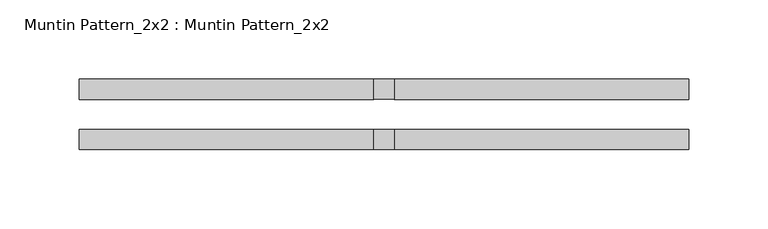
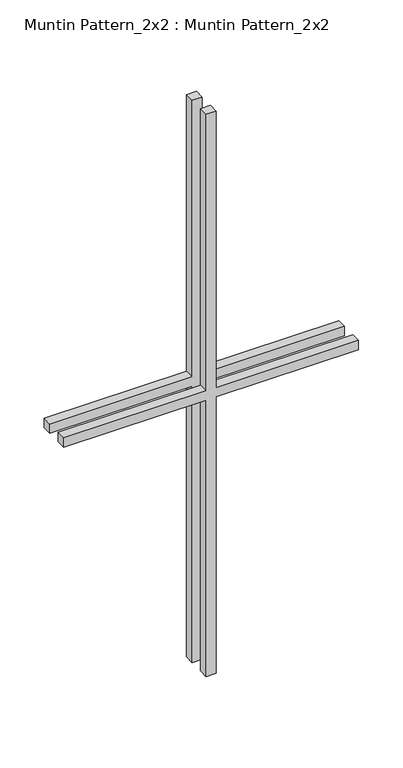
"""IFC4 building model written with IfcOpenShell, lengths in millimetres: proxy geometry, Muntin Pattern_2x2 : Muntin Pattern_2x2."""

from ifc_helpers import new_model, si_unit, frame, origin, place, context, project, spatial, polyline, outline, extrude, source, transform, mapped, element, save


def muntin_pattern_2x2_muntin_pattern_2x2_4af9dbf3(model_context):
    return source(origin(), model_context, "Body", "SweptSolid", [
        extrude(outline(polyline([(393.7, -6.35), (393.7, -192.0875), (381.0, -192.0875), (381.0, -6.35), (0.0, -6.35), (0.0, 6.35), (381.0, 6.35), (381.0, 192.0875), (393.7, 192.0875), (393.7, 6.35), (774.7, 6.35), (774.7, -6.35), (393.7, -6.35)])), frame((0.0, 9.525, 0.0), z_axis=(0.0, 1.0, 0.0), x_axis=(0.0, 0.0, 1.0)), (0.0, 0.0, 1.0), 12.7),
        extrude(outline(polyline([(393.7, -6.35), (393.7, -192.0875), (381.0, -192.0875), (381.0, -6.35), (0.0, -6.35), (0.0, 6.35), (381.0, 6.35), (381.0, 192.0875), (393.7, 192.0875), (393.7, 6.35), (774.7, 6.35), (774.7, -6.35), (393.7, -6.35)])), frame((0.0, -22.225, 0.0), z_axis=(0.0, 1.0, 0.0), x_axis=(0.0, 0.0, 1.0)), (0.0, 0.0, 1.0), 12.7),
    ])


if __name__ == "__main__":
    model = new_model("IFC4")
    model_context = context("Model", 3, world=origin())
    ifc_project = project(units=[si_unit("LENGTHUNIT", "METRE", prefix="MILLI")], contexts=[model_context])
    site = spatial("IfcSite", under=ifc_project)
    building = spatial("IfcBuilding", under=site)
    placement = place(None, origin())
    muntin_pattern_2x2_muntin_pattern_2x2_shape = muntin_pattern_2x2_muntin_pattern_2x2_4af9dbf3(model_context)
    element("IfcBuildingElementProxy", 1, Name="Muntin Pattern_2x2 : Muntin Pattern_2x2", ObjectType="Muntin Pattern_2x2 : Muntin Pattern_2x2", at=placement, inside=building, context=model_context, shape_type="MappedRepresentation", body=[
        mapped(muntin_pattern_2x2_muntin_pattern_2x2_shape, transform((0.0, 0.0, 0.0), x_axis=(1.0, 0.0, 0.0), y_axis=(0.0, 1.0, 0.0), z_axis=(0.0, 0.0, 1.0))),
    ])
    save(model, "model.ifc")

# Revit data of these elements
# Type "Muntin Pattern_2x2 : Muntin Pattern_2x2"
#   Width [instance default] = 4' - 0"
#   Thickness = 0' - 0 1/2"
#   Height [instance default] = 4' - 0"
#   Distance = 0' - 0 3/4"
#   Interior Material [instance default] = none
#   Exterior Material [instance default] = none
#   Default Elevation = 0
# Element 1 (IfcBuildingElementProxy, "Muntin Pattern_2x2 : Muntin Pattern_2x2")
#   Width = 1' - 3 1/8"
#   Height = 2' - 6 1/2"
#   Interior Material = Wood - Stained
#   Exterior Material = Clad - White
#   Materials on its faces: "Clad - White", "Wood - Stained"
# Materials
#   "Clad - White": class "Wood", colour RGB 242 242 238, transparency 0, Cost = 0
#   "Wood - Stained": class "Wood", colour RGB 224 178 126, transparency 0, Cost = 0
